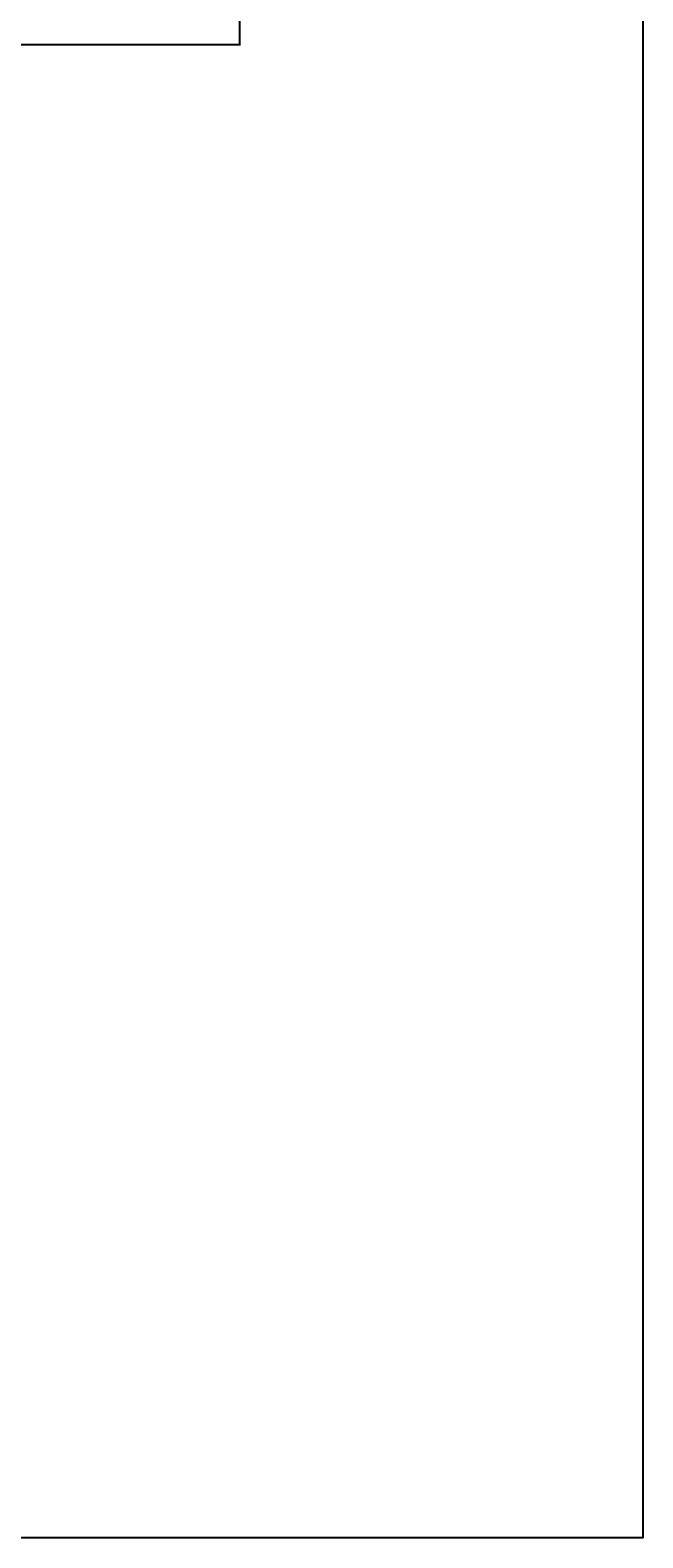
# Model space of a CAD drawing. Units: inches. Extents: x 1770 to 2988, y 1161 to 3221.
# Tile 6 of 44: x 2804 to 2988, y 1161 to 1614. Entities that reach past the tile are written whole.
import ezdxf

# ---------------------------------------------------------------- set-up
doc = ezdxf.new("R2010")
doc.units = ezdxf.units.IN
doc.layers.add('A-ANNO-DIMS', color=2, linetype='Continuous', lineweight=18)
doc.layers.add('A-ANNO-TTLB', color=7, linetype='Continuous', lineweight=25)
doc.styles.get("Standard").update_dxf_attribs({"font": 'arial.ttf'})
doc.dimstyles.get("Standard").update_dxf_attribs({"dimtxt": 0.18, "dimasz": 0.18, "dimexe": 0.18, "dimexo": 0.0625, "dimgap": 0.09, "dimtad": 0, "dimtih": 1, "dimtoh": 1, "dimdec": 4, "dimzin": 0, "dimdsep": 46, "dimtxsty": 'Standard', "dimcen": 0.09, "dimadec": 0, "dimazin": 0, "dimtfac": 1, "dimtdec": 4, "dimtofl": 0, "dimtmove": 0, "dimatfit": 3, "dimfxl": 1, "dimtolj": 1, "dimtzin": 0, "dimarcsym": 0})

# ---------------------------------------------------------------- blocks, each defined once
blk = doc.blocks.new('*D61')
at = {"layer": 'A-ANNO-DIMS', "color": 0, "lineweight": -2, "transparency": 16777216}
for p, q in [((2625.76, 2376.7), (2866.87, 2376.7)), ((2866.69, 2376.52), (2866.69, 1993.63)), ((2866.69, 1610.38), (2866.69, 1993.27)), ((2625.76, 1610.2), (2866.87, 1610.2))]:
    blk.add_line(p, q, dxfattribs=at)
at = {"layer": 'A-ANNO-DIMS', "color": 0, "transparency": 16777216}
for points in [[(2866.66, 2376.52), (2866.72, 2376.52), (2866.69, 2376.7)], [(2866.66, 1610.38), (2866.72, 1610.38), (2866.69, 1610.2)]]:
    blk.add_solid(points, dxfattribs=at)
at = {"layer": 'Defpoints', "color": 0, "transparency": 16777216}
for p in [(2625.7, 2376.7), (2866.69, 2376.7), (2625.7, 1610.2)]:
    blk.add_point(p, dxfattribs=at)
at = {"layer": 'A-ANNO-DIMS', "color": 0, "transparency": 16777216, "insert": (2866.69, 1993.45), "char_height": 0.18, "attachment_point": 5}
blk.add_mtext('\\A1;766.5', dxfattribs=at)

msp = doc.modelspace()

# ---------------------------------------------------------------- linework, layer by layer
at = {"layer": 'A-ANNO-TTLB'}
msp.add_lwpolyline([(1769.9155, 3221.2788), (2987.7567, 3221.2788), (2987.7567, 1161.1516), (1769.9155, 1161.1516)], close=True, dxfattribs=at)

# ---------------------------------------------------------------- dimensions: what is measured, and where the dimension line sits
at = {"layer": 'A-ANNO-DIMS'}
dim = msp.add_linear_dim(base=(2866.6874, 2376.7021), p1=(2625.696, 1610.2021), p2=(2625.696, 2376.7021), angle=90, dimstyle='Standard', override={"dimdec": 1, "dimlfac": 1, "dimrnd": 0, "dimzin": 0, "dimdsep": 46, "dimlunit": 2}, dxfattribs=at)
dim.commit()
dim.dimension.update_dxf_attribs({"geometry": '*D61', "text_midpoint": (2866.6874, 1993.4521)})

doc.saveas('drawing.dxf')
